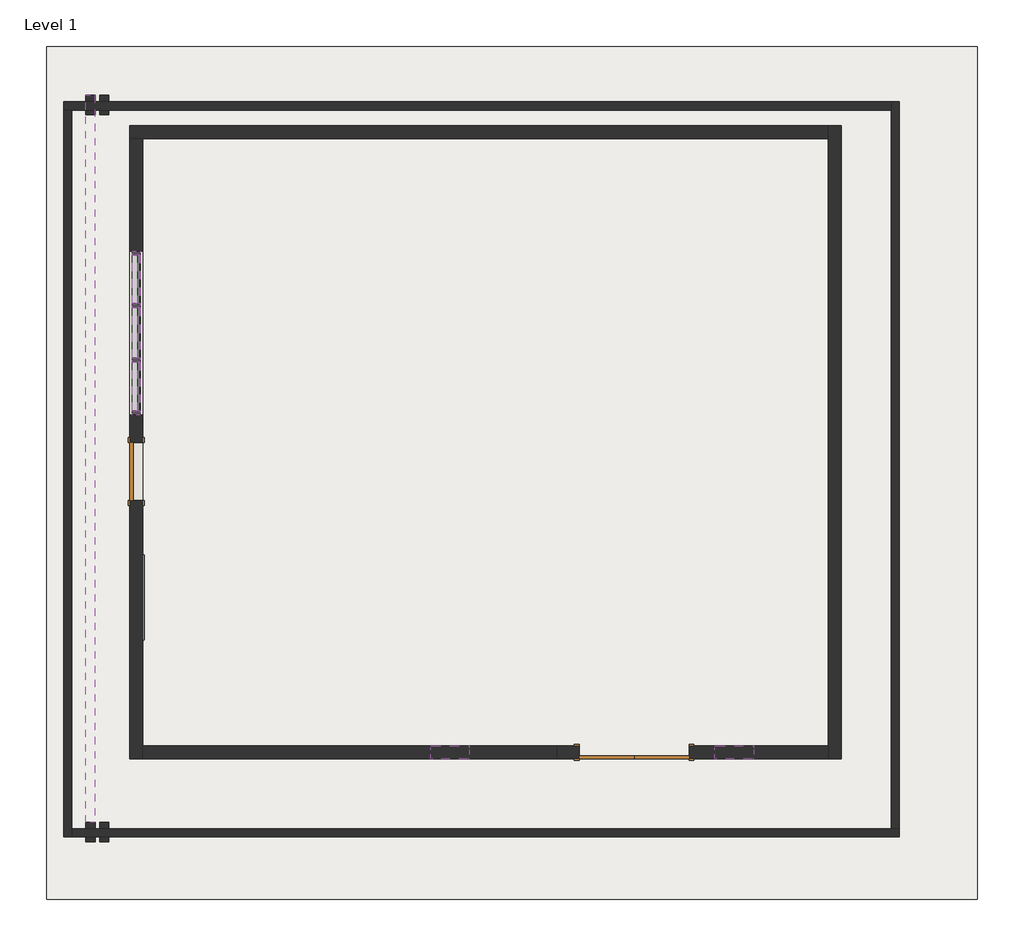
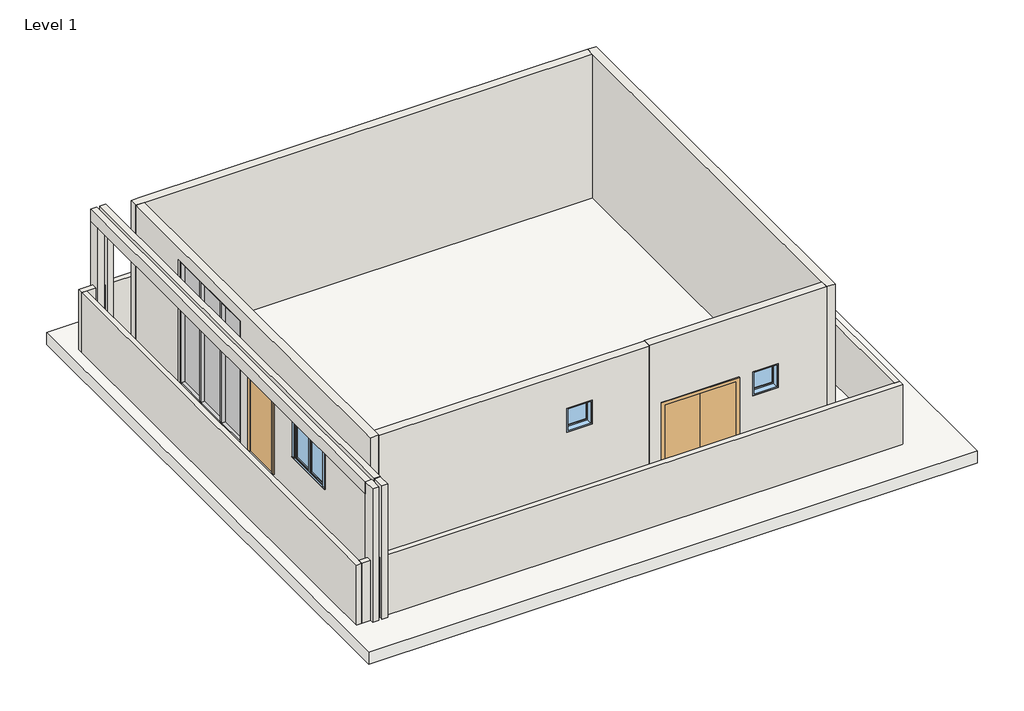
# One storey: 17 members, 12 walls, 6 plates, 3 windows, 2 doors, 1 slab.
"""IFC4 building model written with IfcOpenShell, lengths in millimetres."""

from ifc_helpers import new_model, si_unit, frame, origin, place, context, project, spatial, polyline, outline, extrude, faceted_brep, transform, mapped, element, save
from components import door_aae36eb6, door_4f2f89b6, member_952a807c, member_6afbb202, member_f14326a3, member_2c21e81d, member_a05a67d1, member_6d59fc0e, member_61742b2b, member_aa870034, system_panel_glazed_55ca81fc, system_panel_glazed_973f3ce5, system_panel_glazed_c3295151, system_panel_glazed_82a57ab2, walls_7_walls_7_91501f10, walls_8_walls_7_cfda60ff, walls_9_walls_9_70f34cfa, window_0862ab64, window_6846e476

model = new_model("IFC4")

# Units and contexts
model_context = context("Model", 3, world=origin())
ifc_project = project(units=[si_unit("LENGTHUNIT", "METRE", prefix="MILLI")], contexts=[model_context])

# Site, building, storey
site = spatial("IfcSite", under=ifc_project)
building = spatial("IfcBuilding", under=site)
storey = spatial("IfcBuildingStorey", under=building, Name="Level 1", Elevation=0.0)

# Doors
placement = place(None, origin())
door_shape = door_aae36eb6(model_context)
element("IfcDoor", 1, ObjectType="Door-Double-Flush_Panel : 68\" x 80\"", at=placement, inside=storey, context=model_context, shape_type="MappedRepresentation", body=[
    mapped(door_shape, transform((-3861.4932708, 1502.8609482, 0.0), x_axis=(-1.0, 0.0, 0.0), y_axis=(0.0, -1.0, 0.0), z_axis=(0.0, 0.0, 1.0))),
])
door_2_shape = door_4f2f89b6(model_context)
element("IfcDoor", 2, ObjectType="Single-Flush : 36\" x 80\"", at=placement, inside=storey, context=model_context, shape_type="MappedRepresentation", body=[
    mapped(door_2_shape, transform((-11684.6932708, 5922.4609482, 304.8), x_axis=(0.0, 1.0, 0.0), y_axis=(-1.0, 0.0, 0.0), z_axis=(0.0, 0.0, 1.0))),
])

# Members
member_shape = member_952a807c(model_context)
element("IfcMember", 3, ObjectType="Rectangular Mullion : 2.5\" x 5\" rectangular", at=placement, inside=storey, context=model_context, shape_type="MappedRepresentation", body=[
    mapped(member_shape, transform((-11684.6932708, 7702.5776149, 2590.8), x_axis=(0.0, 0.0, 1.0), y_axis=(-1.0, 0.0, 0.0), z_axis=(0.0, -1.0, 0.0))),
])
member_2_shape = member_6afbb202(model_context)
element("IfcMember", 4, ObjectType="Rectangular Mullion : 2.5\" x 5\" rectangular", at=placement, inside=storey, context=model_context, shape_type="MappedRepresentation", body=[
    mapped(member_2_shape, transform((-11684.6932708, 8530.1942815, 177.8), x_axis=(0.0, -1.0, 0.0), y_axis=(-1.0, 0.0, 0.0), z_axis=(0.0, 0.0, -1.0))),
])
element("IfcMember", 5, ObjectType="Rectangular Mullion : 2.5\" x 5\" rectangular", at=placement, inside=storey, context=model_context, shape_type="MappedRepresentation", body=[
    mapped(member_2_shape, transform((-11684.6932708, 7670.8276149, 177.8), x_axis=(0.0, -1.0, 0.0), y_axis=(-1.0, 0.0, 0.0), z_axis=(0.0, 0.0, -1.0))),
])
member_3_shape = member_f14326a3(model_context)
element("IfcMember", 6, ObjectType="Rectangular Mullion : 2.5\" x 5\" rectangular", at=placement, inside=storey, context=model_context, shape_type="MappedRepresentation", body=[
    mapped(member_3_shape, transform((-11684.6932708, 8498.4442815, 177.8), x_axis=(0.0, 0.0, -1.0), y_axis=(-1.0, 0.0, 0.0), z_axis=(0.0, 1.0, 0.0))),
])
member_4_shape = member_2c21e81d(model_context)
element("IfcMember", 7, ObjectType="Rectangular Mullion : 2.5\" x 5\" rectangular", at=placement, inside=storey, context=model_context, shape_type="MappedRepresentation", body=[
    mapped(member_4_shape, transform((-11684.6932708, 6874.9609482, 2590.8), x_axis=(0.0, 0.0, 1.0), y_axis=(-1.0, 0.0, 0.0), z_axis=(0.0, -1.0, 0.0))),
])
element("IfcMember", 8, ObjectType="Rectangular Mullion : 2.5\" x 5\" rectangular", at=placement, inside=storey, context=model_context, shape_type="MappedRepresentation", body=[
    mapped(member_4_shape, transform((-11684.6932708, 8561.9442815, 2590.8), x_axis=(0.0, 0.0, 1.0), y_axis=(-1.0, 0.0, 0.0), z_axis=(0.0, -1.0, 0.0))),
])
member_5_shape = member_a05a67d1(model_context)
element("IfcMember", 9, ObjectType="Rectangular Mullion : 2.5\" x 5\" rectangular", at=placement, inside=storey, context=model_context, shape_type="MappedRepresentation", body=[
    mapped(member_5_shape, transform((-11684.6932708, 7639.0776149, 177.8), x_axis=(0.0, 0.0, -1.0), y_axis=(-1.0, 0.0, 0.0), z_axis=(0.0, 1.0, 0.0))),
])
element("IfcMember", 10, ObjectType="Rectangular Mullion : 2.5\" x 5\" rectangular", at=placement, inside=storey, context=model_context, shape_type="MappedRepresentation", body=[
    mapped(member_5_shape, transform((-11684.6932708, 9326.0609482, 177.8), x_axis=(0.0, 0.0, -1.0), y_axis=(-1.0, 0.0, 0.0), z_axis=(0.0, 1.0, 0.0))),
])
member_6_shape = member_6d59fc0e(model_context)
element("IfcMember", 11, ObjectType="Rectangular Mullion : 2.5\" x 5\" rectangular", at=placement, inside=storey, context=model_context, shape_type="MappedRepresentation", body=[
    mapped(member_6_shape, transform((-11684.6932708, 9389.5609482, 2590.8), x_axis=(0.0, 1.0, 0.0), y_axis=(-1.0, 0.0, 0.0), z_axis=(0.0, 0.0, 1.0))),
])
element("IfcMember", 12, ObjectType="Rectangular Mullion : 2.5\" x 5\" rectangular", at=placement, inside=storey, context=model_context, shape_type="MappedRepresentation", body=[
    mapped(member_6_shape, transform((-11684.6932708, 6811.4609482, 177.8), x_axis=(0.0, -1.0, 0.0), y_axis=(-1.0, 0.0, 0.0), z_axis=(0.0, 0.0, -1.0))),
])
member_7_shape = member_61742b2b(model_context)
element("IfcMember", 13, ObjectType="Rectangular Mullion : 2.5\" x 5\" rectangular", at=placement, inside=storey, context=model_context, shape_type="MappedRepresentation", body=[
    mapped(member_7_shape, transform((-11684.6932708, 8530.1942815, 2590.8), x_axis=(0.0, -1.0, 0.0), y_axis=(-1.0, 0.0, 0.0), z_axis=(0.0, 0.0, -1.0))),
])
element("IfcMember", 14, ObjectType="Rectangular Mullion : 2.5\" x 5\" rectangular", at=placement, inside=storey, context=model_context, shape_type="MappedRepresentation", body=[
    mapped(member_7_shape, transform((-11684.6932708, 7670.8276149, 2590.8), x_axis=(0.0, -1.0, 0.0), y_axis=(-1.0, 0.0, 0.0), z_axis=(0.0, 0.0, -1.0))),
])
element("IfcMember", 15, ObjectType="Rectangular Mullion : 2.5\" x 5\" rectangular", at=placement, inside=storey, context=model_context, shape_type="MappedRepresentation", body=[
    mapped(member_3_shape, transform((-11684.6932708, 7702.5776149, 3352.8), x_axis=(0.0, 0.0, 1.0), y_axis=(-1.0, 0.0, 0.0), z_axis=(0.0, -1.0, 0.0))),
])
element("IfcMember", 16, ObjectType="Rectangular Mullion : 2.5\" x 5\" rectangular", at=placement, inside=storey, context=model_context, shape_type="MappedRepresentation", body=[
    mapped(member_5_shape, transform((-11684.6932708, 8561.9442815, 3352.8), x_axis=(0.0, 0.0, 1.0), y_axis=(-1.0, 0.0, 0.0), z_axis=(0.0, -1.0, 0.0))),
])
element("IfcMember", 17, ObjectType="Rectangular Mullion : 2.5\" x 5\" rectangular", at=placement, inside=storey, context=model_context, shape_type="MappedRepresentation", body=[
    mapped(member_5_shape, transform((-11684.6932708, 6874.9609482, 3352.8), x_axis=(0.0, 0.0, 1.0), y_axis=(-1.0, 0.0, 0.0), z_axis=(0.0, -1.0, 0.0))),
])
member_8_shape = member_aa870034(model_context)
element("IfcMember", 18, ObjectType="Rectangular Mullion : 2.5\" x 5\" rectangular", at=placement, inside=storey, context=model_context, shape_type="MappedRepresentation", body=[
    mapped(member_8_shape, transform((-11684.6932708, 9389.5609482, 3352.8), x_axis=(0.0, 1.0, 0.0), y_axis=(-1.0, 0.0, 0.0), z_axis=(0.0, 0.0, 1.0))),
])
element("IfcMember", 19, ObjectType="Rectangular Mullion : 2.5\" x 5\" rectangular", at=placement, inside=storey, context=model_context, shape_type="MappedRepresentation", body=[
    mapped(member_8_shape, transform((-11684.6932708, 6811.4609482, 2590.8), x_axis=(0.0, -1.0, 0.0), y_axis=(-1.0, 0.0, 0.0), z_axis=(0.0, 0.0, -1.0))),
])

# Plates
system_panel_glazed_shape = system_panel_glazed_55ca81fc(model_context)
element("IfcPlate", 20, ObjectType="System Panel : Glazed", at=placement, inside=storey, context=model_context, shape_type="MappedRepresentation", body=[
    mapped(system_panel_glazed_shape, transform((-11684.6932708, 8100.5109482, 241.3), x_axis=(0.0, -1.0, 0.0), y_axis=(1.0, 0.0, 0.0), z_axis=(0.0, 0.0, 1.0))),
])
system_panel_glazed_2_shape = system_panel_glazed_973f3ce5(model_context)
element("IfcPlate", 21, ObjectType="System Panel : Glazed", at=placement, inside=storey, context=model_context, shape_type="MappedRepresentation", body=[
    mapped(system_panel_glazed_2_shape, transform((-11684.6932708, 8944.0026149, 241.3), x_axis=(0.0, -1.0, 0.0), y_axis=(1.0, 0.0, 0.0), z_axis=(0.0, 0.0, 1.0))),
])
element("IfcPlate", 22, ObjectType="System Panel : Glazed", at=placement, inside=storey, context=model_context, shape_type="MappedRepresentation", body=[
    mapped(system_panel_glazed_2_shape, transform((-11684.6932708, 7257.0192815, 241.3), x_axis=(0.0, -1.0, 0.0), y_axis=(1.0, 0.0, 0.0), z_axis=(0.0, 0.0, 1.0))),
])
system_panel_glazed_3_shape = system_panel_glazed_c3295151(model_context)
element("IfcPlate", 23, ObjectType="System Panel : Glazed", at=placement, inside=storey, context=model_context, shape_type="MappedRepresentation", body=[
    mapped(system_panel_glazed_3_shape, transform((-11684.6932708, 8944.0026149, 2622.55), x_axis=(0.0, -1.0, 0.0), y_axis=(1.0, 0.0, 0.0), z_axis=(0.0, 0.0, 1.0))),
])
element("IfcPlate", 24, ObjectType="System Panel : Glazed", at=placement, inside=storey, context=model_context, shape_type="MappedRepresentation", body=[
    mapped(system_panel_glazed_3_shape, transform((-11684.6932708, 7257.0192815, 2622.55), x_axis=(0.0, -1.0, 0.0), y_axis=(1.0, 0.0, 0.0), z_axis=(0.0, 0.0, 1.0))),
])
system_panel_glazed_4_shape = system_panel_glazed_82a57ab2(model_context)
element("IfcPlate", 25, ObjectType="System Panel : Glazed", at=placement, inside=storey, context=model_context, shape_type="MappedRepresentation", body=[
    mapped(system_panel_glazed_4_shape, transform((-11684.6932708, 8100.5109482, 2622.55), x_axis=(0.0, -1.0, 0.0), y_axis=(1.0, 0.0, 0.0), z_axis=(0.0, 0.0, 1.0))),
])

# Slab
element("IfcSlab", 26, ObjectType="Generic - 12\"", at=placement, inside=storey, context=model_context, shape_type="SweptSolid", body=[
    extrude(outline(polyline([(1533.7194136, 12604.2670221), (1533.7194136, -806.9329779), (-13096.6805864, -806.9329779), (-13096.6805864, 12604.2670221), (1533.7194136, 12604.2670221)])), frame((0.0, 0.0, -304.8), z_axis=(0.0, 0.0, 1.0), x_axis=(1.0, 0.0, 0.0)), (0.0, 0.0, 1.0), 304.8),
])

# Walls
element("IfcWall", 27, ObjectType="Generic - 5\"", at=placement, inside=storey, context=model_context, shape_type="Brep", body=[
    faceted_brep([(-12827.7867805, 11606.6893426, 0.0), (-12700.7867805, 11606.6893426, 0.0), (177.0132195, 11606.6893426, 0.0), (177.0132195, 11606.6893426, 1524.0), (-12700.7867805, 11606.6893426, 1524.0), (-12827.7867805, 11606.6893426, 1524.0), (-12827.7867805, 11733.6893426, 0.0), (-12827.7867805, 11733.6893426, 1524.0), (177.0132195, 11733.6893426, 1524.0), (177.0132195, 11733.6893426, 0.0)], [[[0, 1, 2, 3, 4, 5]], [[6, 7, 8, 9]], [[2, 1, 0, 6, 9]], [[5, 4, 3, 8, 7]], [[0, 5, 7, 6]], [[3, 2, 9, 8]]]),
])
element("IfcWall", 28, ObjectType="Generic - 5\"", at=placement, inside=storey, context=model_context, shape_type="Brep", body=[
    faceted_brep([(-12700.7867805, 176.6893426, 0.0), (-12700.7867805, 303.6893426, 0.0), (-12700.7867805, 11606.6893426, 0.0), (-12700.7867805, 11606.6893426, 1524.0), (-12700.7867805, 303.6893426, 1524.0), (-12700.7867805, 176.6893426, 1524.0), (-12827.7867805, 176.6893426, 0.0), (-12827.7867805, 176.6893426, 1524.0), (-12827.7867805, 11606.6893426, 1524.0), (-12827.7867805, 11606.6893426, 0.0)], [[[0, 1, 2, 3, 4, 5]], [[6, 7, 8, 9]], [[2, 1, 0, 6, 9]], [[5, 4, 3, 8, 7]], [[0, 5, 7, 6]], [[3, 2, 9, 8]]]),
])
element("IfcWall", 29, ObjectType="Generic - 5\"", at=placement, inside=storey, context=model_context, shape_type="Brep", body=[
    faceted_brep([(304.0132195, 303.6893426, 0.0), (177.0132195, 303.6893426, 0.0), (-12700.7867805, 303.6893426, 0.0), (-12700.7867805, 303.6893426, 1524.0), (177.0132195, 303.6893426, 1524.0), (304.0132195, 303.6893426, 1524.0), (304.0132195, 176.6893426, 0.0), (304.0132195, 176.6893426, 1524.0), (-12700.7867805, 176.6893426, 1524.0), (-12700.7867805, 176.6893426, 0.0)], [[[0, 1, 2, 3, 4, 5]], [[6, 7, 8, 9]], [[2, 1, 0, 6, 9]], [[5, 4, 3, 8, 7]], [[0, 5, 7, 6]], [[3, 2, 9, 8]]]),
])
element("IfcWall", 30, ObjectType="Generic - 5\"", at=placement, inside=storey, context=model_context, shape_type="Brep", body=[
    faceted_brep([(177.0132195, 11733.6893426, 0.0), (177.0132195, 11606.6893426, 0.0), (177.0132195, 303.6893426, 0.0), (177.0132195, 303.6893426, 1524.0), (177.0132195, 11606.6893426, 1524.0), (177.0132195, 11733.6893426, 1524.0), (304.0132195, 11733.6893426, 0.0), (304.0132195, 11733.6893426, 1524.0), (304.0132195, 303.6893426, 1524.0), (304.0132195, 303.6893426, 0.0)], [[[0, 1, 2, 3, 4, 5]], [[6, 7, 8, 9]], [[2, 1, 0, 6, 9]], [[5, 4, 3, 8, 7]], [[0, 5, 7, 6]], [[3, 2, 9, 8]]]),
])
element("IfcWall", 31, ObjectType="Generic - 8\"", at=placement, inside=storey, context=model_context, shape_type="Brep", body=[
    faceted_brep([(-11786.2932708, 11154.8609482, 0.0), (-11583.0932708, 11154.8609482, 0.0), (-813.4932708, 11154.8609482, 0.0), (-813.4932708, 11154.8609482, 3657.6), (-11583.0932708, 11154.8609482, 3657.6), (-11786.2932708, 11154.8609482, 3657.6), (-11786.2932708, 11358.0609482, 0.0), (-11786.2932708, 11358.0609482, 3657.6), (-11583.0932708, 11358.0609482, 3657.6), (-813.4932708, 11358.0609482, 3657.6), (-813.4932708, 11358.0609482, 0.0)], [[[0, 1, 2, 3, 4, 5]], [[6, 7, 8, 9, 10]], [[2, 1, 0, 6, 10]], [[0, 5, 7, 6]], [[2, 10, 9, 3]], [[7, 5, 4, 3, 9, 8]]]),
])
element("IfcWall", 32, ObjectType="Generic - 8\"", at=placement, inside=storey, context=model_context, shape_type="Brep", body=[
    faceted_brep([(-11583.0932708, 1401.2609482, 0.0), (-11583.0932708, 1604.4609482, 0.0), (-11583.0932708, 11154.8609482, 0.0), (-11583.0932708, 11154.8609482, 3657.6), (-11583.0932708, 6811.4609482, 3657.6), (-11583.0932708, 1401.2609482, 3657.6), (-11583.0932708, 1401.2609482, 3648.3275144), (-11583.0932708, 6811.4609482, 3352.8), (-11583.0932708, 9389.5609482, 3352.8), (-11583.0932708, 9389.5609482, 177.8), (-11583.0932708, 6811.4609482, 177.8), (-11583.0932708, 5465.2609482, 304.8), (-11583.0932708, 5465.2609482, 2336.8), (-11583.0932708, 6379.6609482, 2336.8), (-11583.0932708, 6379.6609482, 304.8), (-11583.0932708, 4550.8609482, 2443.0011718), (-11583.0932708, 4550.8609482, 1223.8011718), (-11583.0932708, 3331.6609482, 1223.8011718), (-11583.0932708, 3331.6609482, 2443.0011718), (-11786.2932708, 1401.2609482, 0.0), (-11786.2932708, 1401.2609482, 3657.6), (-11786.2932708, 6786.0609482, 3657.6), (-11786.2932708, 6811.4609482, 3657.6), (-11786.2932708, 11154.8609482, 3657.6), (-11786.2932708, 11154.8609482, 0.0), (-11786.2932708, 6811.4609482, 3352.8), (-11786.2932708, 6811.4609482, 177.8), (-11786.2932708, 9389.5609482, 177.8), (-11786.2932708, 9389.5609482, 3352.8), (-11786.2932708, 5465.2609482, 304.8), (-11786.2932708, 6379.6609482, 304.8), (-11786.2932708, 6379.6609482, 2336.8), (-11786.2932708, 5465.2609482, 2336.8), (-11786.2932708, 4550.8609482, 2443.0011718), (-11786.2932708, 3331.6609482, 2443.0011718), (-11786.2932708, 3331.6609482, 1223.8011718), (-11786.2932708, 4550.8609482, 1223.8011718)], [[[0, 1, 2, 3, 4, 5, 6], [7, 8, 9, 10], [11, 12, 13, 14], [15, 16, 17, 18]], [[19, 20, 21, 22, 23, 24], [25, 26, 27, 28], [29, 30, 31, 32], [33, 34, 35, 36]], [[5, 4, 3, 23, 22, 21, 20]], [[0, 6, 5, 20, 19]], [[2, 1, 0, 19, 24]], [[8, 7, 25, 28]], [[9, 8, 28, 27]], [[10, 9, 27, 26]], [[7, 10, 26, 25]], [[2, 24, 23, 3]], [[30, 29, 11, 14]], [[31, 30, 14, 13]], [[32, 31, 13, 12]], [[29, 32, 12, 11]], [[16, 15, 33, 36]], [[17, 16, 36, 35]], [[18, 17, 35, 34]], [[15, 18, 34, 33]]]),
])
element("IfcWall", 33, ObjectType="Generic - 8\"", at=placement, inside=storey, context=model_context, shape_type="Brep", body=[
    faceted_brep([(-813.4932708, 11358.0609482, 0.0), (-813.4932708, 11154.8609482, 0.0), (-813.4932708, 1604.4609482, 0.0), (-813.4932708, 1401.2609482, 0.0), (-813.4932708, 1401.2609482, 3657.6), (-813.4932708, 1426.6609482, 3657.6), (-813.4932708, 1604.4609482, 3657.6), (-813.4932708, 11154.8609482, 3657.6), (-813.4932708, 11358.0609482, 3657.6), (-610.2932708, 11358.0609482, 0.0), (-610.2932708, 11358.0609482, 3657.6), (-610.2932708, 11154.8609482, 3657.6), (-610.2932708, 1426.6609482, 3657.6), (-610.2932708, 1401.2609482, 3657.6), (-610.2932708, 1401.2609482, 0.0)], [[[0, 1, 2, 3, 4, 5, 6, 7, 8]], [[9, 10, 11, 12, 13, 14]], [[3, 2, 1, 0, 9, 14]], [[0, 8, 10, 9]], [[10, 8, 7, 6, 5, 4, 13, 12, 11]], [[4, 3, 14, 13]]]),
])
element("IfcWall", 34, ObjectType="Generic - 8\"", at=placement, inside=storey, context=model_context, shape_type="SweptSolid", body=[
    extrude(outline(polyline([(0.0, -11583.0932708), (0.0, -5080.6932708), (3648.3275144, -5080.6932708), (3648.3275144, -11583.0932708), (0.0, -11583.0932708)]), holes=[polyline([(2753.9164297, -6452.2932708), (2144.3164297, -6452.2932708), (2144.3164297, -7061.8932708), (2753.9164297, -7061.8932708), (2753.9164297, -6452.2932708)])]), frame((0.0, 1401.2609482, 0.0), z_axis=(0.0, 1.0, 0.0), x_axis=(0.0, 0.0, 1.0)), (0.0, 0.0, 1.0), 203.2),
])
element("IfcWall", 35, ObjectType="Generic - 8\"", at=placement, inside=storey, context=model_context, shape_type="Brep", body=[
    faceted_brep([(-5080.6932708, 1604.4609482, 0.0), (-5080.6932708, 1604.4609482, 3648.3275144), (-5080.6932708, 1604.4609482, 3657.6), (-813.4932708, 1604.4609482, 3657.6), (-813.4932708, 1604.4609482, 0.0), (-2997.8932708, 1604.4609482, 0.0), (-2997.8932708, 1604.4609482, 2032.0), (-4725.0932708, 1604.4609482, 2032.0), (-4725.0932708, 1604.4609482, 0.0), (-1981.8932708, 1604.4609482, 2117.986062), (-2591.4932708, 1604.4609482, 2117.986062), (-2591.4932708, 1604.4609482, 1508.386062), (-1981.8932708, 1604.4609482, 1508.386062), (-5080.6932708, 1401.2609482, 3657.6), (-5080.6932708, 1401.2609482, 3648.3275144), (-5080.6932708, 1401.2609482, 0.0), (-4725.0932708, 1401.2609482, 0.0), (-4725.0932708, 1401.2609482, 2032.0), (-2997.8932708, 1401.2609482, 2032.0), (-2997.8932708, 1401.2609482, 0.0), (-813.4932708, 1401.2609482, 0.0), (-813.4932708, 1401.2609482, 3657.6), (-1981.8932708, 1401.2609482, 2117.986062), (-1981.8932708, 1401.2609482, 1508.386062), (-2591.4932708, 1401.2609482, 1508.386062), (-2591.4932708, 1401.2609482, 2117.986062)], [[[0, 1, 2, 3, 4, 5, 6, 7, 8], [9, 10, 11, 12]], [[13, 14, 15, 16, 17, 18, 19, 20, 21], [22, 23, 24, 25]], [[4, 20, 19, 5]], [[15, 0, 8, 16]], [[2, 1, 0, 15, 14, 13]], [[3, 2, 13, 21]], [[20, 4, 3, 21]], [[7, 17, 16, 8]], [[17, 7, 6, 18]], [[18, 6, 5, 19]], [[23, 22, 9, 12]], [[24, 23, 12, 11]], [[25, 24, 11, 10]], [[22, 25, 10, 9]]]),
])
walls_7_walls_7_shape = walls_7_walls_7_91501f10(model_context)
element("IfcWall", 36, ObjectType="Walls 7 : Walls 7", at=placement, inside=storey, context=model_context, shape_type="MappedRepresentation", body=[
    mapped(walls_7_walls_7_shape, transform((0.0, 0.0, 0.0), x_axis=(1.0, 0.0, 0.0), y_axis=(0.0, 1.0, 0.0), z_axis=(0.0, 0.0, 1.0))),
])
walls_8_walls_7_shape = walls_8_walls_7_cfda60ff(model_context)
element("IfcWall", 37, ObjectType="Walls 8 : Walls 7", at=placement, inside=storey, context=model_context, shape_type="MappedRepresentation", body=[
    mapped(walls_8_walls_7_shape, transform((0.0, 11434.1636015, 0.0), x_axis=(1.0, 0.0, 0.0), y_axis=(0.0, 1.0, 0.0), z_axis=(0.0, 0.0, 1.0))),
])
walls_9_walls_9_shape = walls_9_walls_9_70f34cfa(model_context)
element("IfcWall", 38, ObjectType="Walls 9 : Walls 9", at=placement, inside=storey, context=model_context, shape_type="MappedRepresentation", body=[
    mapped(walls_9_walls_9_shape, transform((0.0, 0.0, 0.0), x_axis=(1.0, 0.0, 0.0), y_axis=(0.0, 1.0, 0.0), z_axis=(0.0, 0.0, 1.0))),
])

# Windows
window_shape = window_0862ab64(model_context)
element("IfcWindow", 39, ObjectType="Casement Dbl with Trim.0001 : 48\" x 48\"", at=placement, inside=storey, context=model_context, shape_type="MappedRepresentation", body=[
    mapped(window_shape, transform((-11665.6432708, 3941.2609482, 309.4011718), x_axis=(0.0, 1.0, 0.0), y_axis=(-1.0, 0.0, 0.0), z_axis=(0.0, 0.0, 1.0))),
])
window_2_shape = window_6846e476(model_context)
element("IfcWindow", 40, ObjectType="Fixed : 24\" x 24\"", at=placement, inside=storey, context=model_context, shape_type="MappedRepresentation", body=[
    mapped(window_2_shape, transform((-6718.9932708, 1502.8609482, 1229.9164297), x_axis=(1.0, 0.0, 0.0), y_axis=(0.0, 1.0, 0.0), z_axis=(0.0, 0.0, 1.0))),
])
element("IfcWindow", 41, ObjectType="Fixed : 24\" x 24\"", at=placement, inside=storey, context=model_context, shape_type="MappedRepresentation", body=[
    mapped(window_2_shape, transform((-2248.5932708, 1502.8609482, 593.986062), x_axis=(1.0, 0.0, 0.0), y_axis=(0.0, 1.0, 0.0), z_axis=(0.0, 0.0, 1.0))),
])

save(model, "model.ifc")

# Revit data of these elements
# Type "Door-Double-Flush_Panel : 68\" x 80\""
#   Type Mark = "9"
#   Construction Type Id = "DOOR"
#   Assembly Code = "C1020"
#   Analytic Construction = "Wooden"
#   Thickness = 0' - 2"
#   Thermal Resistance (R) = 2.5876 (h·ft²·°F)/BTU
#   Swing Angle [instance default] = 90.00°
#   Panel Width = 2' - 10"
#   Heat Transfer Coefficient (U) = 0.3865 BTU/(h·ft²·°F)
#   Height = 6' - 8"
#   Trim Projection Ext = 0' - 1"
#   Trim Projection Int = 0' - 1"
#   Trim Width = 0' - 3"
#   Width = 5' - 8"
#   Define Thermal Properties by = 1
#   Panel Material = Wood - Birch - Solid Stained Light Low Gloss
#   Trim Material = Paint - Sienna
#   Visual Light Transmittance = 0
#   Solar Heat Gain Coefficient = 0
#   Function = (empty or 0)
#   Wall Closure = (empty or 0)
# Type "Single-Flush : 36\" x 80\""
#   Type Mark = "6"
#   Construction Type Id = "MDOOR"
#   Assembly Code = "C1020"
#   Analytic Construction = "Metal"
#   Thickness = 0' - 2"
#   Heat Transfer Coefficient (U) = 0.651978 BTU/(h·ft²·°F)
#   Height = 6' - 8"
#   Trim Projection Ext = 0' - 1"
#   Trim Projection Int = 0' - 1"
#   Trim Width = 0' - 3"
#   Width = 3' - 0"
#   Define Thermal Properties by = 1
#   Door Material = Door - Panel
#   Frame Material = Door - Frame
#   Visual Light Transmittance = 0
#   Solar Heat Gain Coefficient = 0
#   Function = (empty or 0)
#   Wall Closure = (empty or 0)
# Type "Rectangular Mullion : 2.5\" x 5\" rectangular"
#   built-in parameter 1007304 = 0.416667 (stored number, unit not read)
#   built-in parameter 1007301 = 0.104167 (stored number, unit not read)
#   built-in parameter 1007300 = 0.104167 (stored number, unit not read)
# Type "System Panel : Glazed"
#   Construction Type Id = "GSP4R"
#   Analytic Construction = "1/8 in Pilkington single glazing"
#   Visual Light Transmittance = 0.9
#   Solar Heat Gain Coefficient = 0.86
#   Heat Transfer Coefficient (U) = 1.18115 BTU/(h·ft²·°F)
# Type "Generic - 12\""
#   Assembly Code = "B1010"
#   Function = 0
#   Layers, outside or top first: 1' - 0" no material (function 1)
# Type "Generic - 5\""
#   Assembly Code = "B2010"
#   Layers, outside or top first: 0' - 5" no material (function 1)
# Type "Generic - 8\""
#   Assembly Code = "B2010"
#   Layers, outside or top first: 0' - 8" no material (function 1)
# Type "Casement Dbl with Trim.0001 : 48\" x 48\""
#   Type Mark = "10"
#   Construction Type Id = "GSP4R"
#   Assembly Code = "B2020100"
#   Analytic Construction = "1/8 in Pilkington single glazing"
#   Visual Light Transmittance = 0.9
#   Solar Heat Gain Coefficient = 0.78
#   Heat Transfer Coefficient (U) = 0.6496 BTU/(h·ft²·°F)
#   Height = 4' - 0"
#   Default Sill Height = 3' - 0"
#   Trim Projection - Ext. = 0' - 0 1/2"
#   Trim Projection - Int. = 0' - 0 3/4"
#   Trim Width - Exterior = 0' - 3 1/2"
#   Trim Width - Interior = 0' - 3 1/2"
#   Width = 4' - 0"
#   Window Inset = 0' - 0 3/4"
#   Define Thermal Properties by = 1
#   Glass Pane Material = Glass
#   Sash Material = Sash
#   Trim Exterior Material = Trim
#   Trim Interior Material = Trim
#   Wall Closure = (empty or 0)
# Type "Fixed : 24\" x 24\""
#   Type Mark = "3"
#   Construction Type Id = "GSP4R"
#   Assembly Code = "B2020100"
#   Analytic Construction = "1/8 in Pilkington single glazing"
#   Visual Light Transmittance = 0.9
#   Solar Heat Gain Coefficient = 0.78
#   Heat Transfer Coefficient (U) = 0.6496 BTU/(h·ft²·°F)
#   Height = 2' - 0"
#   Default Sill Height = 3' - 0"
#   Width = 2' - 0"
#   Window Inset = 0' - 0 3/4"
#   Define Thermal Properties by = 1
#   Glass Pane Material = Glass
#   Sash Material = Sash
#   Wall Closure = (empty or 0)
# Element 1 (IfcDoor, "Door-Double-Flush_Panel : 68\" x 80\"")
#   Swing Angle = 90.00°
#   Phase Created = New Construction
#   Materials on its faces: "Paint - Sienna", "Wood - Birch - Solid Stained Light Low Gloss"
# Element 2 (IfcDoor, "Single-Flush : 36\" x 80\"")
#   Phase Created = New Construction
#   Materials on its faces: "Door - Frame", "Door - Panel"
# Elements 3, 4, 5, 6, 7, 8, 9, 10, 11, 12, 13, 14, 15, 16, 17, 18, 19 (IfcMember, "Rectangular Mullion : 2.5\" x 5\" rectangular")
#   Phase Created = New Construction
#   Materials on its faces: "Aluminum"
# Elements 20, 21, 22, 23, 24, 25 (IfcPlate, "System Panel : Glazed")
#   Phase Created = New Construction
#   Materials on its faces: "Glass"
# Element 26 (IfcSlab, "Generic - 12\"")
#   Height Offset From Level = 0' - 0"
#   Phase Created = New Construction
#   Materials on its faces: "Default Floor"
# Elements 27, 28, 29, 30 (IfcWall, "Generic - 5\"")
#   Top Offset = -7' - 0"
#   Base Offset = 0' - 0"
#   wall height = 5' - 0"
#   Phase Created = New Construction
#   Base Constraint = Level 1
#   Top Constraint = Level 2
#   Materials on its faces: "Default Wall"
# Elements 31, 32, 33 (IfcWall, "Generic - 8\"")
#   Top Offset = 0' - 0"
#   Base Offset = 0' - 0"
#   Unconnected Height = 20' - 0"
#   wall height = 20' - 0"
#   Phase Created = New Construction
#   Base Constraint = Level 1
#   Materials on its faces: "Default Wall"
# Element 34 (IfcWall, "Generic - 8\"")
#   Top Offset = 0' - 0"
#   Base Offset = 0' - 0"
#   Unconnected Height = 11' - 11.63494"
#   wall height = 11' - 11.63494"
#   Phase Created = New Construction
#   Base Constraint = Level 1
#   Materials on its faces: "Default Wall"
# Element 35 (IfcWall, "Generic - 8\"")
#   Top Offset = 0' - 0"
#   Base Offset = 0' - 0"
#   Unconnected Height = 12' - 0"
#   wall height = 12' - 0"
#   Phase Created = New Construction
#   Base Constraint = Level 1
#   Materials on its faces: "Default Wall"
# Element 36 (IfcWall, "Walls 7 : Walls 7")
#   Phase Created = New Construction
#   Materials on its faces: "Default Wall"
# Element 37 (IfcWall, "Walls 8 : Walls 7")
#   Phase Created = New Construction
#   Materials on its faces: "Default Wall"
# Element 38 (IfcWall, "Walls 9 : Walls 9")
#   Phase Created = New Construction
#   Materials on its faces: "Default Wall"
# Element 39 (IfcWindow, "Casement Dbl with Trim.0001 : 48\" x 48\"")
#   Mark = "1"
#   Phase Created = New Construction
#   Materials on its faces: "Sash", "Trim", "Glass"
# Element 40 (IfcWindow, "Fixed : 24\" x 24\"")
#   Mark = "2"
#   Phase Created = New Construction
#   Materials on its faces: "Sash", "Glass"
# Element 41 (IfcWindow, "Fixed : 24\" x 24\"")
#   Mark = "4"
#   Phase Created = New Construction
#   Materials on its faces: "Sash", "Glass"
# Materials
#   "Wood - Birch - Solid Stained Light Low Gloss": class "Wood", colour RGB 210 159 95, transparency 0, Cost = 0
#   "Paint - Sienna": colour RGB 118 70 51, transparency 0, Cost = 0
#   "Door - Panel": class "Wood", colour RGB 210 159 95, transparency 0
#   "Door - Frame": colour RGB 118 70 51, transparency 0
#   "Glass": class "Glass", colour RGB 0 128 192, transparency 0.75, Description = "Soda Lime Glass", Cost = 0
#   "Sash": class "Wood", colour RGB 224 178 126, transparency 0
#   "Trim": class "Wood", colour RGB 224 178 126, transparency 0
#   "Aluminum": class "Metal", colour RGB 247 247 247, transparency 0, Description = "Aluminum 6061", Cost = 0
#   "Default Floor": colour RGB 128 128 128, transparency 0
#   "Default Wall": colour RGB 128 128 128, transparency 0
